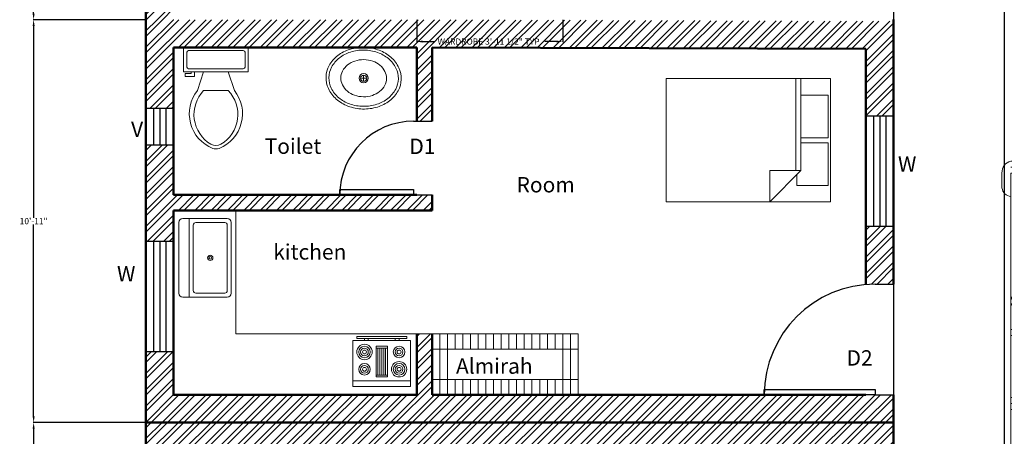
# Model space of a CAD drawing. Units: inches. Extents: x -83 to 408, y 158 to 919.
# Tile 2 of 5: x -82 to 238, y 586 to 721. Entities that reach past the tile are written whole.
import ezdxf

# ---------------------------------------------------------------- set-up
doc = ezdxf.new("R2010")
doc.units = ezdxf.units.IN
doc.header["$MEASUREMENT"] = 0
for name, color, linetype, lineweight in [('A-ANNO-DIMS', 2, 'Continuous', 18), ('A-ANNO-TEXT', 7, 'Continuous', 18), ('A-AREA-IDEN', 7, 'Continuous', 18), ('A-DOOR', 3, 'Continuous', 25), ('A-EQPM', 8, 'Continuous', 18), ('A-FLOR-CASE', 30, 'Continuous', 18), ('A-FLOR-FIXT', 9, 'Continuous', 18), ('A-FURN', 8, 'Continuous', 18), ('A-GLAZ', 4, 'Continuous', 25), ('A-WALL', 7, 'Continuous', 50), ('A-WALL-PATT', 252, 'Continuous', 13), ('C-PKNG-VEHI', 8, 'Continuous', 18)]:
    doc.layers.add(name, color=color, linetype=linetype, lineweight=lineweight)
doc.styles.get("Standard").update_dxf_attribs({"font": 'arial.ttf'})
doc.dimstyles.get("Standard").update_dxf_attribs({"dimtxt": 2, "dimasz": 2, "dimexe": 0.18, "dimexo": 0.0625, "dimgap": 0.09, "dimtad": 0, "dimtih": 1, "dimtoh": 1, "dimdec": 0, "dimzin": 0, "dimdsep": 46, "dimlunit": 3, "dimtxsty": 'Standard', "dimcen": 0.09, "dimadec": 0, "dimazin": 0, "dimtfac": 1, "dimtdec": 0, "dimtofl": 0, "dimtmove": 0, "dimatfit": 3, "dimfxl": 1, "dimtolj": 1, "dimtzin": 0, "dimarcsym": 0})
pattern_1 = [(45, (0, -122.02), (-2.65165, 2.65165), []), (45, (1.7678, -122.02), (-2.65165, 2.65165), [])]

# ---------------------------------------------------------------- blocks, each defined once
blk = doc.blocks.new('Sink - Oval top')
for p, q in [((-1, 0), (1, 0)), ((0, 1), (0, -1))]:
    blk.add_line(p, q)
for points in [[(-12.23, 0.39, 0.117634), (-11.46, -3.36, 0.104469), (-8.88, -6.8, 0.090016), (-5.08, -9.07, 0.08192), (-0.32, -10.02, 0.08192), (4.49, -9.38, 0.090016), (8.42, -7.36, 0.104469), (11.22, -4.09, 0.117634), (12.23, -0.39, 0.117634), (11.46, 3.36, 0.104469), (8.88, 6.8, 0.090016), (5.08, 9.07, 0.08192), (0.32, 10.02, 0.08192), (-4.49, 9.38, 0.090016), (-8.42, 7.36, 0.104469), (-11.22, 4.09, 0.117634)], [(-11.29, 0.16, 0.118622), (-10.52, -3.25, 0.104678), (-8.07, -6.36, 0.089562), (-4.54, -8.37, 0.081185), (-0.13, -9.15, 0.081185), (4.3, -8.49, 0.089562), (7.89, -6.58, 0.104678), (10.42, -3.55, 0.118622), (11.29, -0.16, 0.118622), (10.52, 3.25, 0.104678), (8.07, 6.36, 0.089562), (4.54, 8.37, 0.081185), (0.13, 9.15, 0.081185), (-4.3, 8.49, 0.089562), (-7.89, 6.58, 0.104678), (-10.42, 3.55, 0.118622)], [(-7.42, 0.08, 0.118283), (-6.91, -2.17, 0.104607), (-5.29, -4.21, 0.089718), (-2.97, -5.53, 0.081436), (-0.07, -6.04, 0.081436), (2.84, -5.59, 0.089718), (5.2, -4.33, 0.104607), (6.86, -2.32, 0.118283), (7.42, -0.08, 0.118283), (6.91, 2.17, 0.104607), (5.29, 4.21, 0.089718), (2.97, 5.53, 0.081436), (0.07, 6.04, 0.081436), (-2.84, 5.59, 0.089718), (-5.2, 4.33, 0.104607), (-6.86, 2.32, 0.118283)]]:
    blk.add_lwpolyline(points, format="xyb", close=True)
for radius in [1.5, 1]:
    blk.add_circle((0, 0), radius)
blk = doc.blocks.new('Toilet - top')
for p, q in [((9.5, -6), (9.5, -2)), ((-10, -8.5), (-8, -8.5)), ((-10, -9.5), (-10, -8.5)), ((-7, -9.5), (-10, -9.5)), ((-8, -8.5), (-8, -8)), ((-7, -8), (-7, -9.5)), ((-4, -8), (-6, -14)), ((4, -8), (6, -14)), ((4, -14), (-4, -14))]:
    blk.add_line(p, q)
blk.add_lwpolyline([(10.5, -8), (10.5, 0), (-10.5, 0), (-10.5, -8)], close=True)
for points in [[(-9.5, -2), (-9.5, -6)], [(8.5, -1), (-8.5, -1)], [(-8.5, -7), (8.5, -7)]]:
    blk.add_lwpolyline(points)
for centre, radius, start, end in [((-8.62, -1.88), 0.884, 81.8699, 188.1301), ((8.62, -1.88), 0.884, 351.8699, 98.1301), ((-8.62, -6.12), 0.884, 171.8699, 278.1301), ((8.62, -6.12), 0.884, 261.8699, 8.1301), ((3.52, -21.58), 12.17, 141.4691, 247.9714), ((4.2, -21.82), 11.33, 136.3677, 238.9468), ((-3.52, -21.58), 12.17, 292.0284, 38.5307), ((-4.2, -21.82), 11.33, 301.053, 43.6321), ((0, -27.88), 4, 245.7318, 294.2682), ((0, -29), 4, 254.8605, 285.1395)]:
    blk.add_arc(centre, radius, start, end)
blk = doc.blocks.new('Bed - Queen')
for p, q in [((0, -80.00003), (0, 0)), ((0, 0), (59.99999, 0)), ((59.99999, 0), (59.99999, -80.00003)), ((7.99999, -1.2), (28.79998, -1.2)), ((7.99999, -14.4), (7.99999, -1.2)), ((28.79998, -1.2), (28.79998, -14.4)), ((31.19999, -1.2), (51.99999, -1.2)), ((31.19999, -14.4), (31.19999, -1.2)), ((51.99999, -1.2), (51.99999, -16.4)), ((0, -14.4), (44.8, -14.4)), ((44.8, -16.8), (0, -16.8)), ((59.99999, -29.6), (44.8, -14.4)), ((44.8, -14.4), (44.8, -29.6)), ((51.99999, -16.4), (46.79936, -16.4)), ((44.8, -29.6), (59.99999, -29.6)), ((59.99999, -80.00003), (0, -80.00003))]:
    blk.add_line(p, q)
blk = doc.blocks.new('Sink-single - 30 in top')
blk.add_line((-15, -3.999996), (15, -3.999996))
for points in [[(-13.5, 0), (13.5, 0)], [(-15, -18.499996), (-15, -1.5)], [(15, -1.5), (15, -18.499996)], [(-13.5, -17.499996), (-13.5, -6.499996)], [(-12.5, -5.499996), (12.5, -5.499996)], [(13.5, -6.499996), (13.5, -17.499996)], [(12.5, -18.499996), (-12.5, -18.499996)], [(13.5, -19.999996), (-13.5, -19.999996)]]:
    blk.add_lwpolyline(points)
for radius in [1, 0.5]:
    blk.add_circle((0, -11.999996), radius)
for centre, radius, start, end in [((-13.5, -1.5), 1.5, 90, 180), ((13.5, -1.5), 1.5, 0, 90), ((-12.5, -6.499996), 1, 90, 180), ((12.5, -6.499996), 1, 0, 90), ((-13.5, -18.499996), 1.5, 180, 270), ((-12.5, -17.499996), 1, 180, 270), ((12.5, -17.499996), 1, 270, 0), ((13.5, -18.499996), 1.5, 270, 0)]:
    blk.add_arc(centre, radius, start, end)
blk = doc.blocks.new('Range-Oven - 30 in top')
for p, q in [((0, -3), (30, -3)), ((12, -6), (18, -6)), ((13, -20), (13, -6)), ((14, -6), (14, -20)), ((15, -20), (15, -6)), ((16, -6), (16, -20)), ((17, -20), (17, -6)), ((18, -20), (12, -20)), ((6, -24), (6, -25)), ((8, -25), (8, -24)), ((22, -25), (22, -24)), ((24, -24), (24, -25))]:
    blk.add_line(p, q)
for points in [[(0, -24), (0, 0), (30, 0), (30, -24)], [(12, -21), (12, -5), (18, -5), (18, -21)], [(2, -26), (2, -25), (28, -25), (28, -26)]]:
    blk.add_lwpolyline(points, close=True)
for centre, radius in [((6, -9), 4), ((6, -9), 3), ((6, -9), 2), ((6, -9), 1), ((24, -9), 3), ((24, -9), 2), ((24, -9), 1), ((6, -18), 3), ((24, -18), 4), ((24, -18), 3), ((6, -18), 2), ((6, -18), 1), ((24, -18), 2), ((24, -18), 1)]:
    blk.add_circle(centre, radius)
blk = doc.blocks.new('*U12')
for p, q in [((0, 0), (0, -6)), ((24, 0), (24, -6))]:
    blk.add_line(p, q)
blk.add_lwpolyline([(0, 0), (0, 24), (1.75, 24), (1.75, 0)], close=True)
blk.add_arc((0, 0), 24, 0, 90)
blk = doc.blocks.new('*U13')
for p, q in [((0, 0), (0, -6)), ((36, 0), (36, -6))]:
    blk.add_line(p, q)
blk.add_lwpolyline([(0, 0), (0, 36), (1.75, 36), (1.75, 0)], close=True)
blk.add_arc((0, 0), 36, 0, 90)
blk = doc.blocks.new('*U15')
for p, q in [((5.44, 42.31), (12.12, 42.31)), ((189.69, 42.31), (183.01, 42.31)), ((0.1, -0.41), (0.1, 38.35)), ((2.77, -0.41), (2.77, 38.31)), ((5.44, -0.41), (5.44, 38.24)), ((5.45, 38.31), (16.12, 38.31)), ((16.12, 38.31), (180.34, 38.31)), ((61.52, -0.41), (61.52, 38.31)), ((61.52, 38.31), (77.54, 27.62)), ((64.19, 38.31), (76.2, 30.29)), ((76.2, 30.29), (76.2, 38.31)), ((78.87, 38.31), (78.87, 28.96)), ((106.91, 28.96), (106.91, 38.31)), ((109.58, 27.62), (109.58, 38.31)), ((112.25, 38.31), (112.25, 28.96)), ((140.29, 28.96), (140.29, 38.31)), ((141.62, 27.62), (149.64, 38.31)), ((149.64, -0.41), (149.64, 38.31)), ((189.69, 38.31), (179.01, 38.31)), ((189.69, -0.41), (189.69, 38.24)), ((192.36, -0.41), (192.36, 38.31)), ((195.03, -0.41), (195.03, 38.35)), ((77.54, 27.62), (141.62, 27.62)), ((77.54, -0.41), (77.54, 27.62)), ((78.87, 28.96), (106.91, 28.96)), ((112.25, 28.96), (140.29, 28.96)), ((141.62, -0.41), (141.62, 27.62)), ((5.44, 7.6), (61.52, 15.61)), ((0.1, -0.42), (0.1, -39.18)), ((2.77, -0.41), (2.77, -39.13)), ((5.44, -0.42), (5.44, -39.07)), ((61.52, -0.41), (61.52, -39.13)), ((77.54, -0.41), (77.54, -28.45)), ((141.62, -0.41), (141.62, -28.45)), ((149.64, -0.41), (149.64, -39.13)), ((189.69, -0.42), (189.69, -39.07)), ((192.36, -0.41), (192.36, -39.13)), ((195.03, -0.42), (195.03, -39.18)), ((5.44, -8.42), (61.52, -16.43)), ((61.52, -39.13), (77.54, -28.45)), ((77.54, -28.45), (141.62, -28.45)), ((78.87, -39.13), (78.87, -29.79)), ((78.87, -29.79), (106.91, -29.79)), ((106.91, -29.79), (106.91, -39.13)), ((109.58, -28.45), (109.58, -39.13)), ((112.25, -29.79), (140.29, -29.79)), ((112.25, -39.13), (112.25, -29.79)), ((140.29, -29.79), (140.29, -39.13)), ((141.62, -28.45), (149.64, -39.13)), ((64.19, -39.13), (76.2, -31.12)), ((76.2, -31.12), (76.2, -39.13)), ((5.45, -39.13), (16.12, -39.13)), ((16.12, -39.13), (180.34, -39.13)), ((189.69, -39.13), (179.01, -39.13)), ((5.44, -43.14), (12.12, -43.14)), ((189.69, -43.14), (183.01, -43.14))]:
    blk.add_line(p, q)
for centre, radius, start, end in [((5.06, 37.26), 5.06, 85.6455, 168.0943), ((11.45, 37.64), 4.72, 8.1301, 81.87), ((183.68, 37.64), 4.72, 98.13, 171.8699), ((190.07, 37.26), 5.06, 11.9057, 94.3545), ((5.06, -38.09), 5.06, 191.9057, 274.3545), ((11.45, -38.46), 4.72, 278.13, 351.8699), ((183.68, -38.46), 4.72, 188.1301, 261.87), ((190.07, -38.09), 5.06, 265.6455, 348.0943)]:
    blk.add_arc(centre, radius, start, end)
blk = doc.blocks.new('ALMIRAH-47IN')
for p, q in [((0, 19.88), (47.48, 19.88)), ((0, 19.88), (0, 0)), ((2.48, 19.88), (2.48, 0)), ((4.98, 19.88), (4.98, 0)), ((7.48, 19.88), (7.48, 14.88)), ((9.98, 19.88), (9.98, 14.88)), ((9.98, 19.88), (9.98, 14.88)), ((9.98, 19.88), (9.98, 14.88)), ((12.48, 19.88), (12.48, 14.88)), ((14.98, 19.88), (14.98, 14.88)), ((14.98, 19.88), (14.98, 14.88)), ((17.48, 19.88), (17.48, 14.88)), ((19.98, 19.88), (19.98, 14.88)), ((22.48, 19.88), (22.48, 14.88)), ((22.48, 19.88), (22.48, 14.88)), ((24.98, 19.88), (24.98, 14.88)), ((24.98, 19.88), (24.98, 14.88)), ((27.48, 19.88), (27.48, 14.88)), ((29.98, 19.88), (29.98, 14.88)), ((29.98, 19.88), (29.98, 14.88)), ((29.98, 19.88), (29.98, 14.88)), ((32.48, 19.88), (32.48, 14.88)), ((34.98, 19.88), (34.98, 14.88)), ((37.48, 19.88), (37.48, 14.88)), ((39.98, 19.88), (39.98, 14.88)), ((42.48, 19.88), (42.48, 0)), ((44.98, 19.88), (44.98, 0)), ((47.48, 19.88), (47.48, 0)), ((0, 14.88), (47.48, 14.88)), ((0, 5), (47.48, 5)), ((7.48, 5), (7.48, 0)), ((9.98, 5), (9.98, 0)), ((9.98, 5), (9.98, 0)), ((9.98, 5), (9.98, 0)), ((12.48, 5), (12.48, 0)), ((14.98, 5), (14.98, 0)), ((14.98, 5), (14.98, 0)), ((17.48, 5), (17.48, 0)), ((19.98, 5), (19.98, 0)), ((22.48, 5), (22.48, 0)), ((22.48, 5), (22.48, 0)), ((24.98, 5), (24.98, 0)), ((24.98, 5), (24.98, 0)), ((27.48, 5), (27.48, 0)), ((29.98, 5), (29.98, 0)), ((29.98, 5), (29.98, 0)), ((29.98, 5), (29.98, 0)), ((32.48, 5), (32.48, 0)), ((34.98, 5), (34.98, 0)), ((37.48, 5), (37.48, 0)), ((39.98, 5), (39.98, 0))]:
    blk.add_line(p, q)
blk = doc.blocks.new('WINDOW-36IN')
for p, q in [((2.5, 36), (2.5, 0)), ((4.5, 36), (4.5, 0)), ((6.5, 36), (6.5, 0))]:
    blk.add_line(p, q)
blk.add_lwpolyline([(0, 36), (9, 36), (9, 0), (0, 0)], close=True)
blk = doc.blocks.new('VENT-12IN')
for p, q in [((2.5, 12), (2.5, 0)), ((4.5, 12), (4.5, 0)), ((6.5, 12), (6.5, 0))]:
    blk.add_line(p, q)
blk.add_lwpolyline([(0, 12), (9, 12), (9, 0), (0, 0)], close=True)
blk = doc.blocks.new('COUNTER-L-STUDIO')
for p, q in [((0, 40.12), (0, 40.12)), ((0, 40.12), (0, 0)), ((0, 0), (63.78, 0))]:
    blk.add_line(p, q)
blk = doc.blocks.new('*D37')
at = {"layer": 'A-ANNO-DIMS', "color": 0, "lineweight": -2, "transparency": 16777216}
for p, q in [((47.19, 721.14), (47.19, 713.9)), ((94.67, 721.14), (94.67, 713.9)), ((49.19, 714.08), (52.98, 714.08)), ((92.67, 714.08), (88.88, 714.08))]:
    blk.add_line(p, q, dxfattribs=at)
at = {"layer": 'A-ANNO-DIMS', "color": 0, "transparency": 16777216}
for points in [[(49.19, 714.41), (49.19, 713.75), (47.19, 714.08)], [(92.67, 714.41), (92.67, 713.75), (94.67, 714.08)]]:
    blk.add_solid(points, dxfattribs=at)
at = {"layer": 'Defpoints', "color": 0, "transparency": 16777216}
for p in [(47.19, 721.2), (94.67, 721.2), (94.67, 714.08)]:
    blk.add_point(p, dxfattribs=at)
at = {"layer": 'A-ANNO-DIMS', "color": 0, "transparency": 16777216, "insert": (70.93, 714.08), "char_height": 2, "attachment_point": 5}
blk.add_mtext('\\A1;WARDROBE 3\'-11 1/2" TYP.', dxfattribs=at)
blk = doc.blocks.new('*D42')
at = {"layer": 'A-ANNO-DIMS', "color": 0, "lineweight": -2, "transparency": 16777216}
for p, q in [((-40.87, 843.2), (-77.49, 843.2)), ((-77.31, 841.2), (-77.31, 783.3)), ((-77.31, 723.18), (-77.31, 781.08)), ((-40.87, 721.18), (-77.49, 721.18))]:
    blk.add_line(p, q, dxfattribs=at)
at = {"layer": 'A-ANNO-DIMS', "color": 0, "transparency": 16777216}
for points in [[(-77.64, 841.2), (-76.98, 841.2), (-77.31, 843.2)], [(-77.64, 723.18), (-76.98, 723.18), (-77.31, 721.18)]]:
    blk.add_solid(points, dxfattribs=at)
at = {"layer": 'Defpoints', "color": 0, "transparency": 16777216}
for p in [(-40.81, 843.2), (-77.31, 721.18), (-40.81, 721.18)]:
    blk.add_point(p, dxfattribs=at)
at = {"layer": 'A-ANNO-DIMS', "color": 0, "transparency": 16777216, "insert": (-77.31, 782.19), "char_height": 2, "attachment_point": 5}
blk.add_mtext('\\A1;10\'-2"', dxfattribs=at)
blk = doc.blocks.new('*D43')
at = {"layer": 'A-ANNO-DIMS', "color": 0, "lineweight": -2, "transparency": 16777216}
for p, q in [((-40.87, 721.18), (-77.49, 721.18)), ((-77.31, 719.18), (-77.31, 656.79)), ((-77.31, 592.18), (-77.31, 654.57)), ((-40.87, 590.18), (-77.49, 590.18))]:
    blk.add_line(p, q, dxfattribs=at)
at = {"layer": 'A-ANNO-DIMS', "color": 0, "transparency": 16777216}
for points in [[(-77.64, 719.18), (-76.98, 719.18), (-77.31, 721.18)], [(-77.64, 592.18), (-76.98, 592.18), (-77.31, 590.18)]]:
    blk.add_solid(points, dxfattribs=at)
at = {"layer": 'Defpoints', "color": 0, "transparency": 16777216}
for p in [(-40.81, 721.18), (-77.31, 590.18), (-40.81, 590.18)]:
    blk.add_point(p, dxfattribs=at)
at = {"layer": 'A-ANNO-DIMS', "color": 0, "transparency": 16777216, "insert": (-77.31, 655.68), "char_height": 2, "attachment_point": 5}
blk.add_mtext('\\A1;10\'-11"', dxfattribs=at)
blk = doc.blocks.new('*D44')
at = {"layer": 'A-ANNO-DIMS', "color": 0, "lineweight": -2, "transparency": 16777216}
for p, q in [((-40.87, 590.18), (-77.49, 590.18)), ((-77.31, 588.18), (-77.31, 525.79)), ((-77.31, 461.18), (-77.31, 523.57)), ((-40.87, 459.18), (-77.49, 459.18))]:
    blk.add_line(p, q, dxfattribs=at)
at = {"layer": 'A-ANNO-DIMS', "color": 0, "transparency": 16777216}
for points in [[(-77.64, 588.18), (-76.98, 588.18), (-77.31, 590.18)], [(-77.64, 461.18), (-76.98, 461.18), (-77.31, 459.18)]]:
    blk.add_solid(points, dxfattribs=at)
at = {"layer": 'Defpoints', "color": 0, "transparency": 16777216}
for p in [(-40.81, 590.18), (-77.31, 459.18), (-40.81, 459.18)]:
    blk.add_point(p, dxfattribs=at)
at = {"layer": 'A-ANNO-DIMS', "color": 0, "transparency": 16777216, "insert": (-77.31, 524.68), "char_height": 2, "attachment_point": 5}
blk.add_mtext('\\A1;10\'-11"', dxfattribs=at)
blk = doc.blocks.new('*D59')
at = {"layer": 'A-ANNO-DIMS', "color": 0, "lineweight": -2, "transparency": 16777216}
for p, q in [((202.19, 769.53), (202.19, 160.47)), ((238.19, 769.53), (238.19, 160.47)), ((204.19, 160.65), (217.44, 160.65)), ((236.19, 160.65), (222.94, 160.65))]:
    blk.add_line(p, q, dxfattribs=at)
at = {"layer": 'A-ANNO-DIMS', "color": 0, "transparency": 16777216}
for points in [[(204.19, 160.98), (204.19, 160.32), (202.19, 160.65)], [(236.19, 160.98), (236.19, 160.32), (238.19, 160.65)]]:
    blk.add_solid(points, dxfattribs=at)
at = {"layer": 'Defpoints', "color": 0, "transparency": 16777216}
for p in [(202.19, 769.59), (238.19, 769.59), (238.19, 160.65)]:
    blk.add_point(p, dxfattribs=at)
at = {"layer": 'A-ANNO-DIMS', "color": 0, "transparency": 16777216, "insert": (220.19, 160.65), "char_height": 2, "attachment_point": 5}
blk.add_mtext('\\A1;3\'-0"', dxfattribs=at)

msp = doc.modelspace()

# ---------------------------------------------------------------- hatches: boundary and pattern name
at = {"layer": 'A-WALL-PATT'}
h = msp.add_hatch(dxfattribs=at)
h.set_pattern_fill('ANSI32', color=256, scale=10)
h.paths.add_polyline_path([(202.19, 842.67), (52.21, 843.2), (-40.81, 843.2), (-40.81, 814.39), (-31.81, 814.39), (-31.81, 834.2), (47.19, 834.2), (47.19, 810.2), (52.19, 810.2), (52.19, 834.2), (193.19, 833.7), (193.19, 811.95), (202.19, 811.95)])
h.paths.add_polyline_path([(-31.81, 781.2), (52.19, 781.2), (52.19, 786.2), (46.19, 786.2), (22.19, 786.2), (-31.81, 786.2), (-31.81, 802.39), (-40.81, 802.39), (-40.81, 771.16), (-31.81, 771.16)])
h.paths.add_polyline_path([(-31.81, 735.16), (-40.81, 735.16), (-40.81, 721.18), (-31.81, 721.18)])
h.paths.add_polyline_path([(202.19, 775.95), (193.19, 775.95), (193.19, 757.08, -0.020861), (196.19, 757.2), (202.19, 757.2)])
h = msp.add_hatch(dxfattribs=at)
h.set_pattern_fill('ANSI32', color=256, scale=10)
h.set_pattern_definition(pattern_1)
h.paths.add_polyline_path([(202.19, 720.65), (52.21, 721.18), (-40.81, 721.18), (-40.81, 692.37), (-31.81, 692.37), (-31.81, 712.18), (47.19, 712.18), (47.19, 688.18), (52.19, 688.18), (52.19, 712.18), (193.19, 711.68), (193.19, 689.93), (202.19, 689.93)])
h.paths.add_polyline_path([(202.19, 653.93), (193.19, 653.93), (193.19, 635.05, -0.020861), (196.19, 635.18), (202.19, 635.18)])
h.paths.add_polyline_path([(202.19, 599.18), (196.19, 599.18), (160.19, 599.18), (52.19, 599.18), (52.19, 619.06), (47.19, 619.06), (47.19, 599.18), (-31.81, 599.18), (-31.81, 613.14), (-40.81, 613.14), (-40.81, 590.18), (202.19, 590.18)])
h.paths.add_polyline_path([(52.19, 664.18), (46.19, 664.18), (22.19, 664.18), (-31.81, 664.18), (-31.81, 680.37), (-40.81, 680.37), (-40.81, 649.14), (-31.81, 649.14), (-31.81, 659.18), (52.19, 659.18)])
h = msp.add_hatch(dxfattribs=at)
h.set_pattern_fill('ANSI32', color=256, scale=10)
h.set_pattern_definition(pattern_1)
h.paths.add_polyline_path([(202.19, 459.71), (52.21, 459.18), (-40.81, 459.18), (-40.81, 487.99), (-31.81, 487.99), (-31.81, 468.18), (47.19, 468.18), (47.19, 492.18), (52.19, 492.18), (52.19, 468.18), (193.19, 468.68), (193.19, 490.43), (202.19, 490.43)])
h.paths.add_polyline_path([(202.19, 526.43), (193.19, 526.43), (193.19, 545.31, 0.020861), (196.19, 545.18), (202.19, 545.18)])
h.paths.add_polyline_path([(202.19, 581.18), (196.19, 581.18), (160.19, 581.18), (52.19, 581.18), (52.19, 561.3), (47.19, 561.3), (47.19, 581.18), (-31.81, 581.18), (-31.81, 567.22), (-40.81, 567.22), (-40.81, 590.18), (202.19, 590.18)])
h.paths.add_polyline_path([(52.19, 516.18), (46.19, 516.18), (22.19, 516.18), (-31.81, 516.18), (-31.81, 499.99), (-40.81, 499.99), (-40.81, 531.22), (-31.81, 531.22), (-31.81, 521.18), (52.19, 521.18)])

# ---------------------------------------------------------------- linework, layer by layer
at = {"layer": 'A-WALL'}
for p, q in [((-40.81, 712.2), (-40.81, 843.2)), ((-40.81, 590.18), (-40.81, 721.18)), ((202.19, 712.2), (202.19, 721.2)), ((202.19, 635.18), (202.19, 720.65)), ((-31.81, 712.18), (47.19, 712.18)), ((-31.81, 664.18), (-31.81, 712.18)), ((47.19, 712.18), (47.19, 688.18)), ((52.19, 712.18), (52.19, 688.18)), ((193.19, 711.68), (52.19, 712.18)), ((52.19, 712.18), (52.19, 688.18)), ((193.19, 635.05), (193.19, 711.68)), ((47.19, 664.18), (-31.81, 664.18)), ((-31.81, 664.18), (47.19, 664.18)), ((52.19, 664.18), (52.19, 659.18)), ((52.19, 664.18), (52.19, 659.18)), ((47.19, 659.18), (-31.81, 659.18)), ((-31.81, 659.18), (52.19, 659.18)), ((-31.81, 599.18), (-31.81, 659.18)), ((47.19, 619.06), (47.19, 599.18)), ((52.19, 619.06), (52.19, 599.18)), ((47.19, 599.18), (-31.81, 599.18)), ((52.19, 599.18), (193.19, 599.18)), ((202.19, 590.18), (202.19, 599.18)), ((-40.81, 590.18), (202.19, 590.18)), ((-40.81, 590.18), (-40.81, 459.18)), ((-40.81, 590.18), (202.19, 590.18)), ((202.19, 590.18), (202.19, 581.18))]:
    msp.add_line(p, q, dxfattribs=at)

# ---------------------------------------------------------------- block references
at = {"layer": 'A-DOOR', "rotation": 90}
for name, p in [('*U12', (46.19, 664.18)), ('*U13', (196.19, 599.18))]:
    msp.add_blockref(name, p, dxfattribs=at)
at = {"layer": 'A-EQPM', "xscale": 0.6253442555691314, "yscale": 0.6253442555691314, "zscale": 0.6253442555691314, "rotation": 180}
msp.add_blockref('Range-Oven - 30 in top', (45.23, 601.86), dxfattribs=at)
at = {"layer": 'A-FLOR-CASE'}
for name, p in [('COUNTER-L-STUDIO', (-11.59, 619.06)), ('ALMIRAH-47IN', (52.19, 599.18))]:
    msp.add_blockref(name, p, dxfattribs=at)
at = {"layer": 'A-FLOR-FIXT'}
for name, p in [('Toilet - top', (-18.06, 712.18)), ('Sink - Oval top', (29.95, 702.16))]:
    msp.add_blockref(name, p, dxfattribs=at)
at = {"layer": 'A-FLOR-FIXT', "xscale": 0.8513407291768876, "yscale": 0.8513407291768876, "zscale": 0.8513407291768876, "rotation": 90}
msp.add_blockref('Sink-single - 30 in top', (-30.11, 643.73), dxfattribs=at)
at = {"layer": 'A-FURN', "xscale": 0.667678018977486, "yscale": 0.667678018977486, "zscale": 0.667678018977486, "rotation": 270}
msp.add_blockref('Bed - Queen', (181.69, 702.02), dxfattribs=at)
at = {"layer": 'A-GLAZ'}
for name, p in [('VENT-12IN', (-40.81, 680.37)), ('WINDOW-36IN', (193.19, 653.93)), ('WINDOW-36IN', (-40.81, 613.14))]:
    msp.add_blockref(name, p, dxfattribs=at)
at = {"layer": 'C-PKNG-VEHI', "xscale": 0.7198545955529133, "yscale": 0.7198545955529133, "zscale": 0.7198545955529133, "rotation": 270}
msp.add_blockref('*U15', (268.48, 675.24), dxfattribs=at)

# ---------------------------------------------------------------- texts
at = {"layer": 'A-ANNO-TEXT', "char_height": 5, "attachment_point": 1}
for s, width, insert in [('V', 4.2263, (-45.64, 688.05)), ('D1', 13.3697, (44.82, 682.5)), ('W', 4.9358, (203.62, 676.74)), ('W', 4.9358, (-50.22, 641.06)), ('Almirah', 24.1185, (59.97, 611.04)), ('D2', 13.3697, (186.91, 613.69))]:
    msp.add_mtext_dynamic_manual_height_columns(s, width=width, gutter_width=1, heights=[0], dxfattribs=dict(at, insert=insert))
at = {"layer": 'A-AREA-IDEN', "char_height": 5, "attachment_point": 1}
for s, width, heights, insert in [('Toilet', 21.3997, [0.203], (-2.22, 682.55)), ('Room', 29.7735, [0], (79.66, 670.01)), ('kitchen', 18.1432, [0], (0.57, 648.17))]:
    msp.add_mtext_dynamic_manual_height_columns(s, width=width, gutter_width=1, heights=heights, dxfattribs=dict(at, insert=insert))

# ---------------------------------------------------------------- dimensions: what is measured, and where the dimension line sits
at = {"layer": 'A-ANNO-DIMS'}
for base, p1, p2, picture, middle in [((-77.31, 721.18), (-40.81, 843.2), (-40.81, 721.18), '*D42', (-77.31, 782.19)), ((-77.31, 590.18), (-40.81, 721.18), (-40.81, 590.18), '*D43', (-77.31, 655.68)), ((-77.31, 459.18), (-40.81, 590.18), (-40.81, 459.18), '*D44', (-77.31, 524.68))]:
    dim = msp.add_linear_dim(base=base, p1=p1, p2=p2, angle=90, dimstyle='Standard', override={"dimdec": 1, "dimlfac": 1, "dimrnd": 0, "dimzin": 1, "dimdsep": 46, "dimlunit": 4, "dimfrac": 2}, dxfattribs=at)
    dim.commit()
    dim.dimension.update_dxf_attribs({"geometry": picture, "text_midpoint": middle})
dim = msp.add_linear_dim(base=(238.19, 160.65), p1=(202.19, 769.59), p2=(238.19, 769.59), dimstyle='Standard', override={"dimdec": 1, "dimlfac": 1, "dimrnd": 0, "dimzin": 1, "dimdsep": 46, "dimlunit": 4, "dimfrac": 2}, dxfattribs=at)
dim.commit()
dim.dimension.update_dxf_attribs({"geometry": '*D59', "text_midpoint": (220.19, 160.65)})
dim = msp.add_linear_dim(base=(94.67, 714.08), p1=(47.19, 721.2), p2=(94.67, 721.2), text='WARDROBE <> TYP.', dimstyle='Standard', override={"dimdec": 1, "dimlfac": 1, "dimrnd": 0, "dimzin": 1, "dimdsep": 46, "dimlunit": 4, "dimfrac": 2}, dxfattribs=at)
dim.commit()
dim.dimension.update_dxf_attribs({"geometry": '*D37', "text_midpoint": (70.93, 714.08)})

doc.saveas('drawing.dxf')
